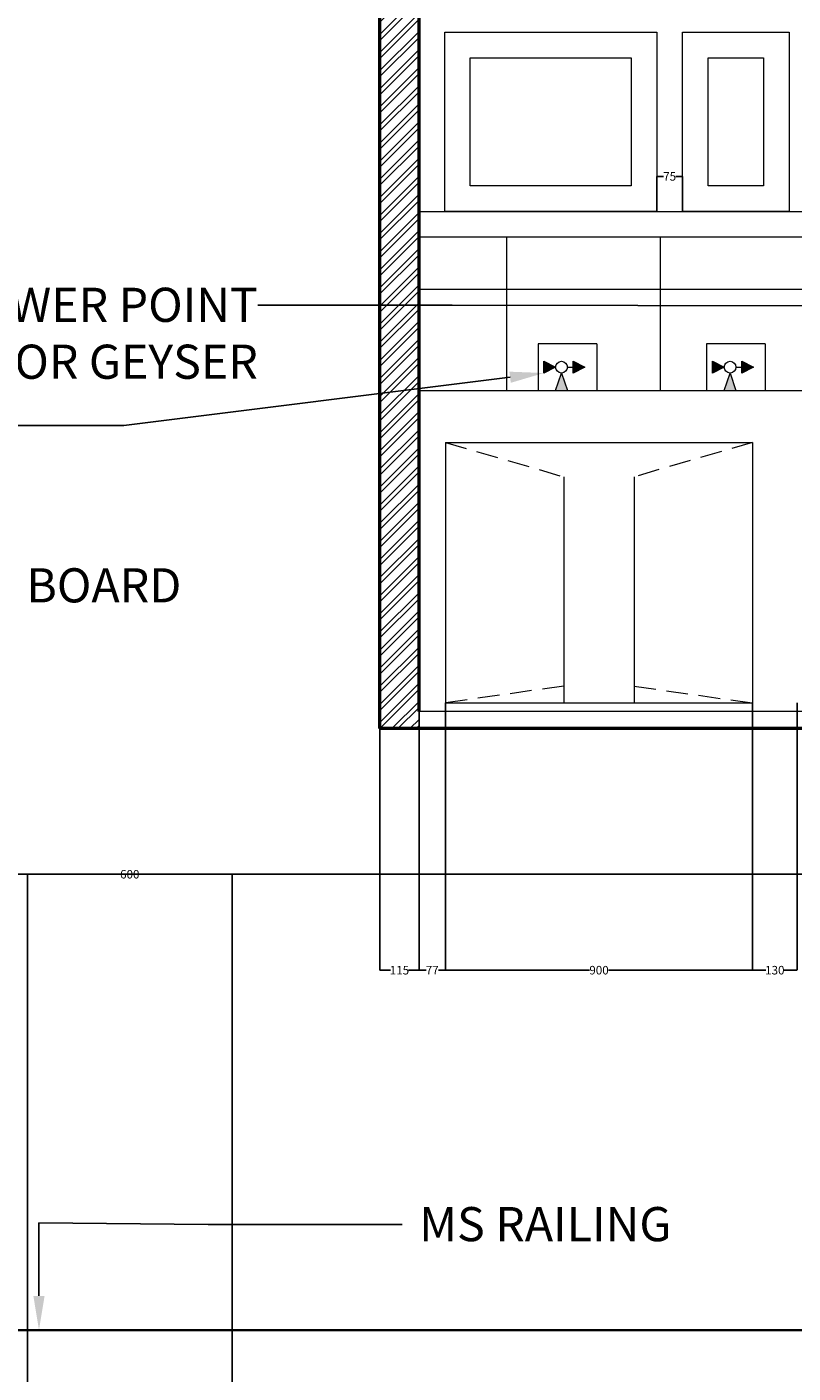
# Model space of a CAD drawing. Units: millimetres. Extents: x 1944 to 29915, y -10550 to 5909.
# Tile 14 of 24: x 11743 to 13987, y -1857 to 2086. Entities that reach past the tile are written whole.
import ezdxf
from ezdxf import colors
from ezdxf.entities.mleader import LeaderData, LeaderLine
from ezdxf.math import Vec2, Vec3

# ---------------------------------------------------------------- set-up
doc = ezdxf.new("R2010")
doc.units = ezdxf.units.MM
doc.header["$MEASUREMENT"] = 0
doc.linetypes.add('HIDDEN', pattern=[9.525, 6.35, -3.175])
for name, color, linetype, lineweight in [('A-ANNO-DIMS', 2, 'Continuous', 18), ('A-ANNO-TEXT', 7, 'Continuous', 25), ('A-ELEV', 3, 'Continuous', 18), ('A-ELEV-HIDN', 3, 'HIDDEN', 13), ('A-SECT', 7, 'Continuous', 35), ('A-WALL', 7, 'Continuous', 50), ('A-WALL-PATT', 8, 'Continuous', 18), ('P-FIXT', 6, 'Continuous', 18)]:
    doc.layers.add(name, color=color, linetype=linetype, lineweight=lineweight)
doc.styles.get("Standard").update_dxf_attribs({"font": 'arial.ttf'})
doc.dimstyles.get("Standard").update_dxf_attribs({"dimtxt": 25, "dimasz": 0.18, "dimexe": 0.18, "dimexo": 0.0625, "dimgap": 0.09, "dimtad": 0, "dimtih": 1, "dimtoh": 1, "dimdec": 0, "dimzin": 0, "dimdsep": 46, "dimtxsty": 'Standard', "dimcen": 0.09, "dimadec": 0, "dimazin": 0, "dimtfac": 1, "dimtdec": 0, "dimtofl": 0, "dimtmove": 0, "dimatfit": 3, "dimfxl": 1, "dimtolj": 1, "dimtzin": 0, "dimarcsym": 0})

# ---------------------------------------------------------------- blocks, each defined once
blk = doc.blocks.new('*D7')
at = {"layer": 'A-ANNO-DIMS', "color": 0, "lineweight": -2, "transparency": 16777216}
for p, q in [((13588, 1545.7), (13588, 1648.2)), ((13588.2, 1648), (13607.6, 1648)), ((13662.9, 1648), (13643.5, 1648)), ((13663, 1545.7), (13663, 1648.2))]:
    blk.add_line(p, q, dxfattribs=at)
at = {"layer": 'A-ANNO-DIMS', "color": 0, "transparency": 16777216}
for points in [[(13588.2, 1648), (13588.2, 1648), (13588, 1648)], [(13662.9, 1648), (13662.9, 1648), (13663, 1648)]]:
    blk.add_solid(points, dxfattribs=at)
at = {"layer": 'Defpoints', "color": 0, "transparency": 16777216}
for p in [(13663, 1648), (13588, 1545.7), (13663, 1545.7)]:
    blk.add_point(p, dxfattribs=at)
at = {"layer": 'A-ANNO-DIMS', "color": 0, "transparency": 16777216, "insert": (13625.5, 1648), "char_height": 25, "attachment_point": 5}
blk.add_mtext('\\A1;75', dxfattribs=at)
blk = doc.blocks.new('Valve - Servo')
for p, q in [((0, 0.2), (-0.5, 0.2)), ((-0.5, 0.2), (-0.5, -0.2)), ((-0.45, -0.05), (-0.45, 0.05)), ((-0.45, 0.05), (-0.350001, 0)), ((-0.350001, 0), (-0.45, -0.05)), ((-0.25, 0), (-0.2, 0)), ((-0.2, -0.05), (-0.2, 0.05)), ((-0.2, 0.05), (-0.1, 0)), ((-0.1, 0), (-0.2, -0.05)), ((-0.350001, -0.2), (-0.3, -0.05)), ((-0.3, -0.05), (-0.25, -0.2)), ((-0.5, -0.2), (0, -0.2))]:
    blk.add_line(p, q)
blk.add_circle((-0.3, 0), 0.05)
for points in [[(-0.45, 0.05), (-0.45, -0.05), (-0.350001, 0)], [(-0.2, 0.05), (-0.1, 0), (-0.2, -0.05)], [(-0.3, -0.05), (-0.350001, -0.2), (-0.25, -0.2)]]:
    blk.add_solid(points)
blk = doc.blocks.new('*D63')
at = {"layer": 'A-ANNO-DIMS', "color": 0, "lineweight": -2, "transparency": 16777216}
for p, q in [((12776.5, 30.8), (12776.5, -677)), ((12891.5, 30.8), (12891.5, -677)), ((12776.7, -676.8), (12807.4, -676.8)), ((12891.4, -676.8), (12860.7, -676.8))]:
    blk.add_line(p, q, dxfattribs=at)
at = {"layer": 'A-ANNO-DIMS', "color": 0, "transparency": 16777216}
for points in [[(12776.7, -676.8), (12776.7, -676.9), (12776.5, -676.8)], [(12891.4, -676.8), (12891.4, -676.9), (12891.5, -676.8)]]:
    blk.add_solid(points, dxfattribs=at)
at = {"layer": 'Defpoints', "color": 0, "transparency": 16777216}
for p in [(12776.5, 30.8), (12891.5, 30.8), (12891.5, -676.8)]:
    blk.add_point(p, dxfattribs=at)
at = {"layer": 'A-ANNO-DIMS', "color": 0, "transparency": 16777216, "insert": (12834, -676.8), "char_height": 25, "attachment_point": 5}
blk.add_mtext('\\A1;115', dxfattribs=at)
blk = doc.blocks.new('*D64')
at = {"layer": 'A-ANNO-DIMS', "color": 0, "lineweight": -2, "transparency": 16777216}
for p, q in [((12891.5, 81), (12891.5, -677)), ((12968.5, 105.8), (12968.5, -677)), ((12891.7, -676.8), (12912.2, -676.8)), ((12968.4, -676.8), (12947.9, -676.8))]:
    blk.add_line(p, q, dxfattribs=at)
at = {"layer": 'A-ANNO-DIMS', "color": 0, "transparency": 16777216}
for points in [[(12891.7, -676.8), (12891.7, -676.9), (12891.5, -676.8)], [(12968.4, -676.8), (12968.4, -676.9), (12968.5, -676.8)]]:
    blk.add_solid(points, dxfattribs=at)
at = {"layer": 'Defpoints', "color": 0, "transparency": 16777216}
for p in [(12891.5, 81), (12968.5, 105.8), (12968.5, -676.8)]:
    blk.add_point(p, dxfattribs=at)
at = {"layer": 'A-ANNO-DIMS', "color": 0, "transparency": 16777216, "insert": (12930, -676.8), "char_height": 25, "attachment_point": 5}
blk.add_mtext('\\A1;77', dxfattribs=at)
blk = doc.blocks.new('*D65')
at = {"layer": 'A-ANNO-DIMS', "color": 0, "lineweight": -2, "transparency": 16777216}
for p, q in [((12968.5, 105.8), (12968.5, -677)), ((13868.5, 105.8), (13868.5, -677)), ((12968.7, -676.8), (13390.9, -676.8)), ((13868.4, -676.8), (13446.2, -676.8))]:
    blk.add_line(p, q, dxfattribs=at)
at = {"layer": 'A-ANNO-DIMS', "color": 0, "transparency": 16777216}
for points in [[(12968.7, -676.8), (12968.7, -676.9), (12968.5, -676.8)], [(13868.4, -676.8), (13868.4, -676.9), (13868.5, -676.8)]]:
    blk.add_solid(points, dxfattribs=at)
at = {"layer": 'Defpoints', "color": 0, "transparency": 16777216}
for p in [(12968.5, 105.8), (13868.5, 105.8), (13868.5, -676.8)]:
    blk.add_point(p, dxfattribs=at)
at = {"layer": 'A-ANNO-DIMS', "color": 0, "transparency": 16777216, "insert": (13418.5, -676.8), "char_height": 25, "attachment_point": 5}
blk.add_mtext('\\A1;900', dxfattribs=at)
blk = doc.blocks.new('*D66')
at = {"layer": 'A-ANNO-DIMS', "color": 0, "lineweight": -2, "transparency": 16777216}
for p, q in [((13868.5, 105.8), (13868.5, -677)), ((13998.5, 105.8), (13998.5, -677)), ((13868.7, -676.8), (13907.1, -676.8)), ((13998.4, -676.8), (13960, -676.8))]:
    blk.add_line(p, q, dxfattribs=at)
at = {"layer": 'A-ANNO-DIMS', "color": 0, "transparency": 16777216}
for points in [[(13868.7, -676.8), (13868.7, -676.9), (13868.5, -676.8)], [(13998.4, -676.8), (13998.4, -676.9), (13998.5, -676.8)]]:
    blk.add_solid(points, dxfattribs=at)
at = {"layer": 'Defpoints', "color": 0, "transparency": 16777216}
for p in [(13868.5, 105.8), (13998.5, 105.8), (13998.5, -676.8)]:
    blk.add_point(p, dxfattribs=at)
at = {"layer": 'A-ANNO-DIMS', "color": 0, "transparency": 16777216, "insert": (13933.5, -676.8), "char_height": 25, "attachment_point": 5}
blk.add_mtext('\\A1;130', dxfattribs=at)
blk = doc.blocks.new('*D85')
at = {"layer": 'A-ANNO-DIMS', "color": 0, "lineweight": -2, "transparency": 16777216}
for p, q in [((6418.3, -1730.7), (6418.3, -395.6)), ((6418.5, -395.8), (15860.3, -395.8)), ((25389.1, -395.8), (15947.3, -395.8)), ((25389.3, -1846.5), (25389.3, -395.6))]:
    blk.add_line(p, q, dxfattribs=at)
at = {"layer": 'A-ANNO-DIMS', "color": 0, "transparency": 16777216}
for points in [[(6418.5, -395.7), (6418.5, -395.8), (6418.3, -395.8)], [(25389.1, -395.7), (25389.1, -395.8), (25389.3, -395.8)]]:
    blk.add_solid(points, dxfattribs=at)
at = {"layer": 'Defpoints', "color": 0, "transparency": 16777216}
for p in [(25389.3, -395.8), (6418.3, -1730.8), (25389.3, -1846.5)]:
    blk.add_point(p, dxfattribs=at)
at = {"layer": 'A-ANNO-DIMS', "color": 0, "transparency": 16777216, "insert": (15903.8, -395.8), "char_height": 25, "attachment_point": 5}
blk.add_mtext('\\A1;18971', dxfattribs=at)
blk = doc.blocks.new('*D93')
at = {"layer": 'A-ANNO-DIMS', "color": 0, "lineweight": -2, "transparency": 16777216}
for p, q in [((11744, -5171.4), (11744, -395.6)), ((11744.2, -395.8), (12016.2, -395.8)), ((12343.8, -395.8), (12071.7, -395.8)), ((12344, -5171.4), (12344, -395.6))]:
    blk.add_line(p, q, dxfattribs=at)
at = {"layer": 'A-ANNO-DIMS', "color": 0, "transparency": 16777216}
for points in [[(11744.2, -395.7), (11744.2, -395.8), (11744, -395.8)], [(12343.8, -395.7), (12343.8, -395.8), (12344, -395.8)]]:
    blk.add_solid(points, dxfattribs=at)
at = {"layer": 'Defpoints', "color": 0, "transparency": 16777216}
for p in [(12344, -395.8), (11744, -5171.5), (12344, -5171.5)]:
    blk.add_point(p, dxfattribs=at)
at = {"layer": 'A-ANNO-DIMS', "color": 0, "transparency": 16777216, "insert": (12044, -395.8), "char_height": 25, "attachment_point": 5}
blk.add_mtext('\\A1;600', dxfattribs=at)

msp = doc.modelspace()

# ---------------------------------------------------------------- hatches: boundary and pattern name
at = {"layer": 'A-WALL-PATT'}
h = msp.add_hatch(dxfattribs=at)
h.set_pattern_fill('ANSI32', color=256, scale=100)
h.paths.add_polyline_path([(12891.548, 3230.657), (12776.548, 3230.657), (12776.548, 30.837), (12891.548, 30.837)])

# ---------------------------------------------------------------- linework, layer by layer
at = {"layer": 'A-ELEV'}
for p, q in [((12891.548, 1545.657), (16975.67, 1545.657)), ((12891.548, 1470.657), (16975.67, 1470.657)), ((13148.195, 1020.657), (13148.195, 1470.657)), ((13598.906, 1020.657), (13598.906, 1470.657)), ((12891.548, 1317.451), (15525.455, 1317.451)), ((13411.687, 1158.026), (13411.687, 1020.657)), ((13905.52, 1158.026), (13905.52, 1020.657)), ((12891.548, 1020.657), (16975.67, 1020.657)), ((12968.548, 868.657), (12968.548, 105.837)), ((12968.548, 868.657), (13868.548, 868.657)), ((13868.548, 868.657), (13868.548, 105.657)), ((13315.349, 768.181), (13315.349, 105.837)), ((13521.747, 768.181), (13521.747, 105.837)), ((16975.67, 81.017), (12891.548, 81.017)), ((12968.548, 105.837), (13868.548, 105.837)), ((12891.548, 30.837), (16975.67, 30.837)), ((12968.548, 30.657), (13868.548, 30.657)), ((13868.548, 30.837), (13868.548, 30.657))]:
    msp.add_line(p, q, dxfattribs=at)
for points in [[(12966.548, 2070.657), (13588.047, 2070.657), (13588.047, 1545.657), (12966.548, 1545.657)], [(13663.047, 2070.657), (13975.393, 2070.657), (13975.393, 1545.657), (13663.047, 1545.657)], [(13041.548, 1995.657), (13513.047, 1995.657), (13513.047, 1620.657), (13041.548, 1620.657)], [(13738.047, 1995.657), (13900.393, 1995.657), (13900.393, 1620.657), (13738.047, 1620.657)]]:
    msp.add_lwpolyline(points, close=True, dxfattribs=at)
at = {"layer": 'A-ELEV-HIDN', "ltscale": 10}
for p, q in [((12968.548, 868.657), (13315.349, 768.181)), ((13868.548, 868.657), (13521.747, 768.181)), ((13315.349, 155.321), (12968.548, 105.837)), ((13521.747, 155.141), (13868.548, 105.657))]:
    msp.add_line(p, q, dxfattribs=at)
at = {"layer": 'A-SECT'}
msp.add_line((6418.315, -1730.752), (16516.552, -1730.752), dxfattribs=at)
at = {"layer": 'A-WALL'}
for p, q in [((12776.548, 30.837), (12776.548, 3230.657)), ((12891.548, 81.017), (12891.548, 3230.657)), ((24504.139, 30.837), (12776.548, 30.837))]:
    msp.add_line(p, q, dxfattribs=at)

# ---------------------------------------------------------------- block references
at = {"layer": 'P-FIXT', "xscale": 343.4227580400382, "yscale": 343.4227580400382, "zscale": 343.4227580400382}
for p in [(13411.687, 1089.342), (13905.52, 1089.342)]:
    msp.add_blockref('Valve - Servo', p, dxfattribs=at)

# ---------------------------------------------------------------- dimensions: what is measured, and where the dimension line sits
at = {"layer": 'A-ANNO-DIMS'}
for base, p1, p2, override, picture, middle in [((13663.047, 1648.015), (13588.047, 1545.657), (13663.047, 1545.657), {"dimclrd": 0, "dimclre": 0, "dimclrt": 0}, '*D7', (13625.547, 1648.015)), ((12968.548, -676.843), (12891.548, 81.017), (12968.548, 105.837), {"dimdec": 0, "dimlfac": 1, "dimrnd": 0, "dimzin": 0, "dimdsep": 46, "dimlunit": 2}, '*D64', (12930.048, -676.843)), ((13868.548, -676.843), (12968.548, 105.837), (13868.548, 105.837), {"dimdec": 0, "dimlfac": 1, "dimrnd": 0, "dimzin": 0, "dimdsep": 46, "dimlunit": 2}, '*D65', (13418.548, -676.843)), ((13998.548, -676.843), (13868.548, 105.837), (13998.548, 105.837), {"dimdec": 0, "dimlfac": 1, "dimrnd": 0, "dimzin": 0, "dimdsep": 46, "dimlunit": 2}, '*D66', (13933.548, -676.843)), ((12891.548, -676.843), (12776.548, 30.837), (12891.548, 30.837), {"dimdec": 0, "dimlfac": 1, "dimrnd": 0, "dimzin": 0, "dimdsep": 46, "dimlunit": 2}, '*D63', (12834.048, -676.843)), ((25389.297, -395.752), (6418.315, -1730.752), (25389.297, -1846.542), {"dimdec": 0, "dimlfac": 1, "dimrnd": 0, "dimzin": 0, "dimdsep": 46, "dimlunit": 2}, '*D85', (15903.806, -395.752)), ((12343.981, -395.752), (11743.981, -5171.512), (12343.981, -5171.512), {"dimdec": 0, "dimlfac": 1, "dimrnd": 0, "dimzin": 0, "dimdsep": 46, "dimlunit": 2}, '*D93', (12043.981, -395.752))]:
    dim = msp.add_linear_dim(base=base, p1=p1, p2=p2, dimstyle='Standard', override=override, dxfattribs=at)
    dim.commit()
    dim.dimension.update_dxf_attribs({"geometry": picture, "text_midpoint": middle})

# ---------------------------------------------------------------- leaders
at = {"layer": 'A-ANNO-TEXT'}
ml = msp.add_multileader_mtext('Standard', dxfattribs=at)
ml.set_content('15 AMP POWER POINT \\PFOR GEYSER ', color=256)
ml.set_leader_properties()
ml.build(insert=Vec2(0, 0))
ml.multileader.update_dxf_attribs({"dogleg_length": 0.36, "arrow_head_size": 100})
ctx = ml.context
ctx.base_point, ctx.char_height, ctx.arrow_head_size, ctx.landing_gap_size, ctx.plane_origin = Vec3(10908.052, 1271.067), 100, 100, 0.09, Vec3(12988.354, 1271.067)
ctx.text_align_type = 2
notes = []
notes.append((ctx, [(0, (1, 1, 0), (12988.354, 1271.067), (-1, 0), 568.936, [(0, [(14591.122, 1267.898)], 0, [])])]))
ctx.mtext.insert, ctx.mtext.alignment, ctx.mtext.flow_direction = Vec3(12419.329, 1321.919), 3, 5
ml = msp.add_multileader_mtext('Standard', dxfattribs=at)
ml.set_content('TAP', color=256)
ml.set_leader_properties()
ml.build(insert=Vec2(0, 0))
ml.multileader.update_dxf_attribs({"dogleg_length": 568.936, "arrow_head_size": 100})
ctx = ml.context
ctx.base_point, ctx.char_height, ctx.arrow_head_size, ctx.landing_gap_size, ctx.plane_origin = Vec3(11195.309, 918.379), 100, 100, 0.09, Vec3(12026.771, 918.379)
ctx.text_align_type = 2
notes.append((ctx, [(0, (1, 1, 0), (12026.771, 918.379), (-1, 0), 568.936, [(0, [(13257.147, 1072.171)], 0, [])])]))
ctx.mtext.insert, ctx.mtext.alignment, ctx.mtext.flow_direction = Vec3(11457.746, 968.379), 3, 5
ml = msp.add_multileader_mtext('Standard', dxfattribs=at)
ml.set_content('SWITCH BOARD', color=256)
ml.set_leader_properties()
ml.build(insert=Vec2(0, 0))
ml.multileader.update_dxf_attribs({"dogleg_length": 568.936, "arrow_head_size": 100})
ctx = ml.context
ctx.base_point, ctx.char_height, ctx.arrow_head_size, ctx.landing_gap_size, ctx.plane_origin = Vec3(11122.176, 449.474), 100, 100, 0.09, Vec3(10553.24, 449.474)
ctx.text_align_type = 2
notes.append((ctx, [(0, (1, 1, 0), (10553.24, 449.474), (1, 0), 568.936, [(0, [(8914.665, 260.837), (8914.665, 449.474)], 0, [])])]))
ctx.mtext.insert, ctx.mtext.alignment, ctx.mtext.flow_direction = Vec3(12195.117, 500.327), 3, 5
ml = msp.add_multileader_mtext('Standard', dxfattribs=at)
ml.set_content('MS RAILING', color=256)
ml.set_leader_properties()
ml.build(insert=Vec2(0, 0))
ml.multileader.update_dxf_attribs({"dogleg_length": 568.936, "arrow_head_size": 100})
ctx = ml.context
ctx.base_point, ctx.char_height, ctx.arrow_head_size, ctx.landing_gap_size, ctx.plane_origin = Vec3(12842.355, -1421.356), 100, 100, 0.09, Vec3(12273.42, -1421.356)
ctx.text_align_type = 2
notes.append((ctx, [(0, (1, 1, 0), (12273.42, -1421.356), (1, 0), 568.936, [(0, [(11778.035, -1730.752), (11778.035, -1416.503)], 0, [])])]))
ctx.mtext.insert, ctx.mtext.alignment, ctx.mtext.flow_direction = Vec3(13630.645, -1370.503), 3, 5
for ctx, leaders in notes:
    for number, flags, end, landing, length, lines in leaders:
        leader = LeaderData()
        leader.index, (leader.has_last_leader_line, leader.has_dogleg_vector, leader.attachment_direction) = number, flags
        leader.last_leader_point, leader.dogleg_vector, leader.dogleg_length = Vec3(end), Vec3(landing), length
        for number, points, colour, breaks in lines:
            line = LeaderLine()
            line.index, line.vertices, line.color, line.breaks = number, Vec3.list(points), colors.encode_raw_color(colour), breaks
            leader.lines.append(line)
        ctx.leaders.append(leader)

doc.saveas('drawing.dxf')
